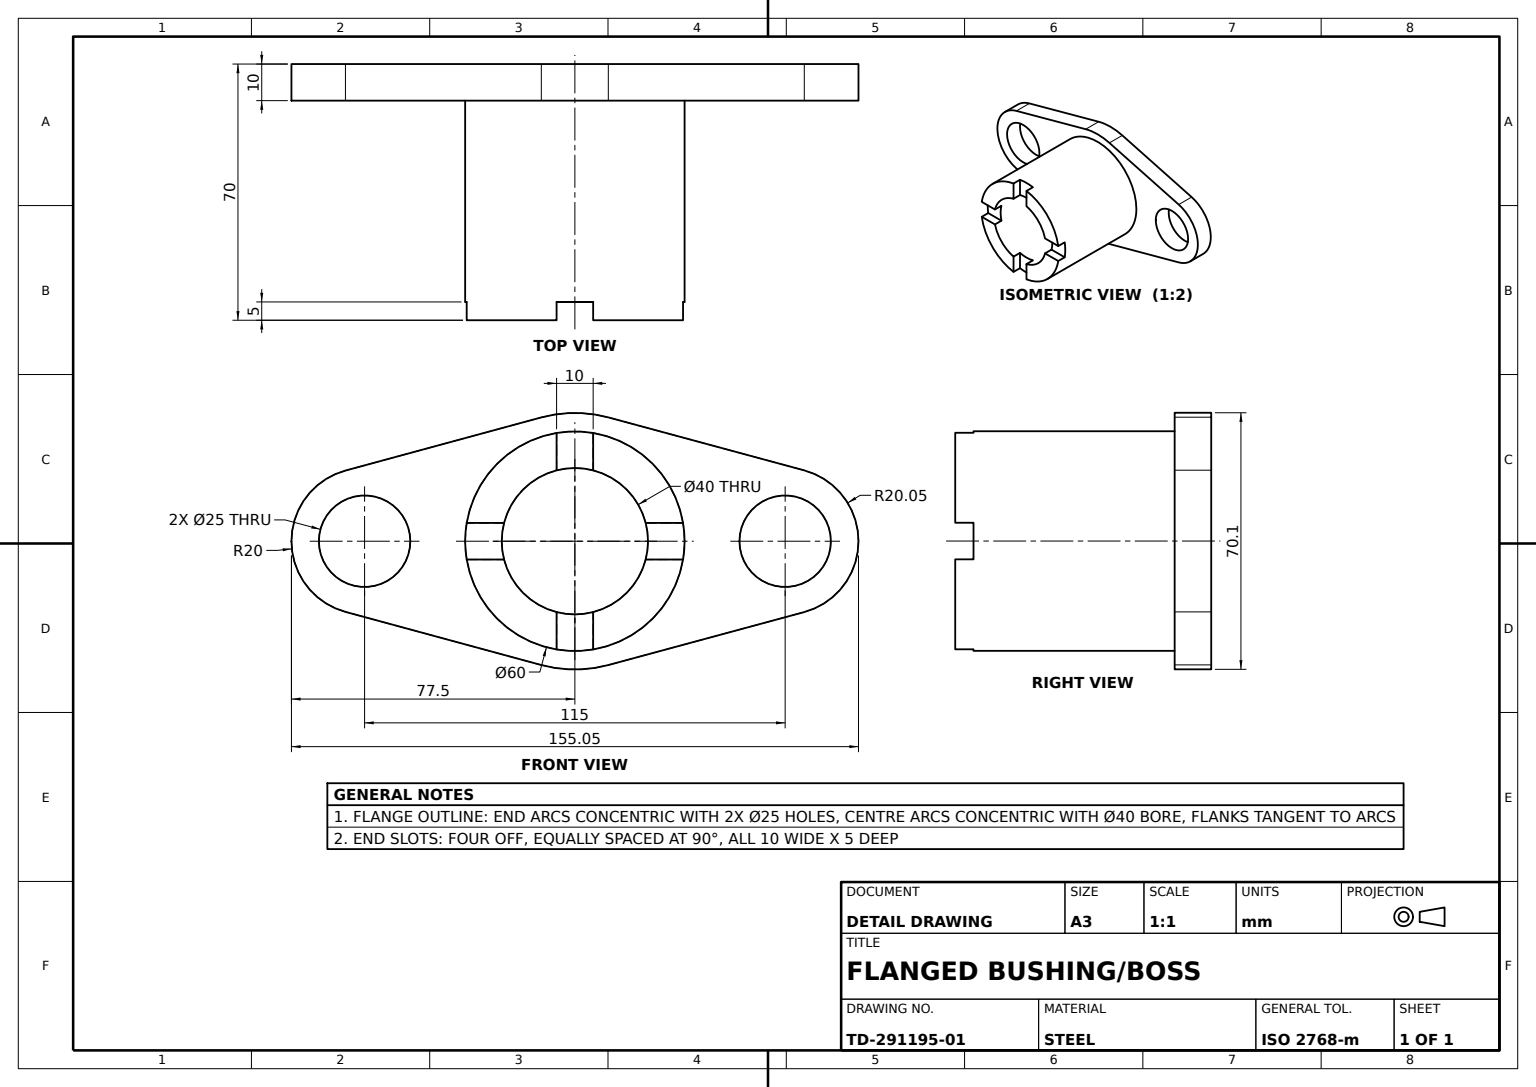
SolidWorks part; units mm, degrees
material "Plain Carbon Steel"
ref_plane "Front Plane" through (0, 0, 0) normal (0, 0, 1) x (1, 0, 0)
ref_plane "Top Plane" through (0, 0, 0) normal (0, 1, 0) x (1, 0, 0)
ref_plane "Right Plane" through (0, 0, 0) normal (1, 0, 0) x (0, 0, -1)
sketch "Flange Plate Sketch" plane through (0, 0, 0) normal (0, 0, 1) x (1, 0, 0)
  line L0 (0, 0) -> (-57.5, 0)
  line L1 (0, 0) -> (57.5, 0)
  line L4 (9.1438, 33.8373) -> (62.7307, 19.3566)
  line L5 (9.1438, -33.8373) -> (62.7307, -19.3566)
  line L6 (-62.7351, 19.3025) -> (-9.1749, 33.8288)
  line L7 (-62.7351, -19.3025) -> (-9.1749, -33.8288)
  arc A0 (-62.7351, 19.3025) -> (-62.7351, -19.3025) centre (-57.5, 0) ccw
  arc A1 (62.7307, -19.3566) -> (62.7307, 19.3566) centre (57.5, 0) ccw
  arc A2 (-9.1749, -33.8288) -> (9.1438, -33.8373) centre (0, 0) ccw
  arc A3 (9.1438, 33.8373) -> (-9.1749, 33.8288) centre (0, 0) ccw
  dimension "D3" = 35.051
  dimension "D1" = 115
  dimension "D2" = 57.5
  dimension "D4" = 55.509
  dimension "D5" = 55.4952
extrude "Flange Plate" add sketch "Flange Plate Sketch" along normal blind 10
sketch "Cylinder Boss Sketch" plane through (0, 0, 10) normal (0, 0, 1) x (1, 0, 0)
  circle A0 centre (0, 0) radius 30
  dimension "D1" = 60
extrude "Cylinder Boss" add sketch "Cylinder Boss Sketch" along normal blind 60
sketch "Bore Sketch" plane through (0, 0, 70) normal (0, 0, 1) x (1, 0, 0)
  circle A0 centre (0, 0) radius 20
  dimension "D1" = 40
extrude "Through Bore" cut sketch "Bore Sketch" against normal blind 70
sketch "End Slots Sketch" plane through (0, 0, 70) normal (0, 0, 1) x (1, 0, 0)
  line L0 (0, 0) -> (0, 30)
  line L1 (0, 30) -> (-5, 30)
  line L2 (-5, 30) -> (5, 30)
  line L3 (5, 30) -> (5, 17.3606)
  line L4 (5, 17.3606) -> (-5, 17.3606)
  line L5 (-5, 17.3606) -> (-5, 30)
  line L6 (0, 0) -> (0, -30)
  line L7 (0, -30) -> (5, -30)
  line L8 (5, -30) -> (5, -16.7191)
  line L9 (5, -16.7191) -> (-5, -16.7191)
  line L10 (0, -30) -> (-5, -30)
  line L11 (-5, -30) -> (-5, -16.7191)
  line L12 (0, 0) -> (-30, 0)
  line L13 (-30, 0) -> (30, 0)
  line L14 (-30, 0) -> (-30, 5)
  line L15 (-30, 5) -> (-30, -5)
  line L16 (-30, -5) -> (-14.5483, -5)
  line L17 (-14.5483, -5) -> (-14.5483, 5)
  line L18 (-14.5483, 5) -> (-30, 5)
  line L19 (30, 0) -> (30, 5)
  line L20 (30, 5) -> (30, -5)
  line L21 (30, -5) -> (17.3498, -5)
  line L22 (17.3498, -5) -> (17.3498, 5)
  line L23 (17.3498, 5) -> (30, 5)
  circle A0 centre (0, 0) radius 30 construction
  circle A1 centre (0, 0) radius 30 construction
  circle A2 centre (0, 0) radius 20 construction
  dimension "D1" = 5
  dimension "D2" = 17.3498
  dimension "D3" = 14.5483
  dimension "D4" = 17.3606
  dimension "D5" = 16.7191
extrude "End Slots 4x" cut sketch "End Slots Sketch" against normal blind 5
sketch "Mounting Holes Sketch" plane through (0, 0, 10) normal (0, 0, 1) x (1, 0, 0)
  circle A0 centre (-57.5, 0) radius 12.5
  circle A1 centre (57.5, 0) radius 12.5
  dimension "D1" = 25
extrude "Mounting Holes 2x" cut sketch "Mounting Holes Sketch" against normal blind 10
